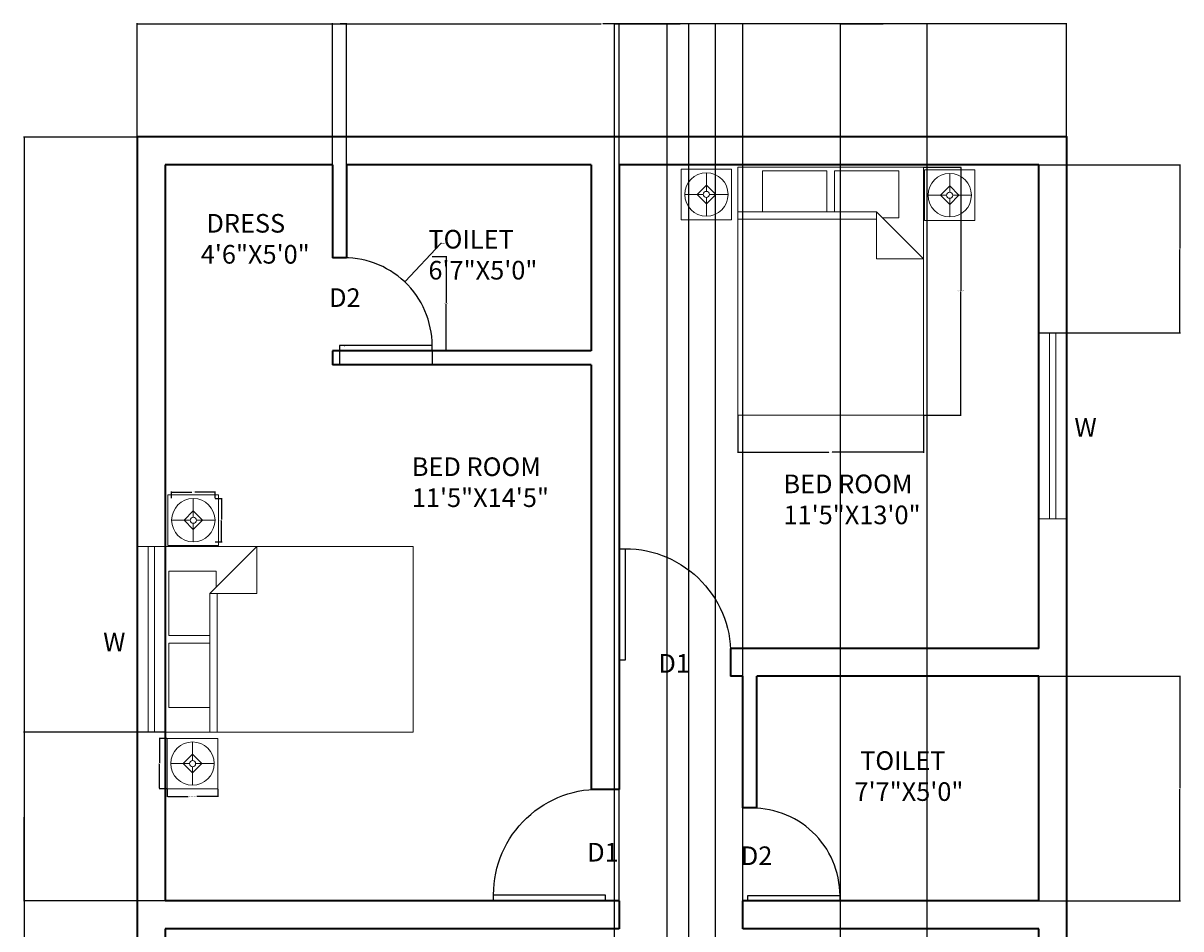
# Model space of a CAD drawing. Units: inches. Extents: x 2523 to 5630, y 2079 to 4208.
# Tile 3 of 3: x 2523 to 2897, y 2520 to 2812. Entities that reach past the tile are written whole.
import ezdxf

# ---------------------------------------------------------------- set-up
doc = ezdxf.new("R2010")
doc.units = ezdxf.units.IN
for name, color, linetype, lineweight in [('A-ANNO-DIMS', 2, 'Continuous', 18), ('A-ANNO-TEXT', 7, 'Continuous', 18), ('A-AREA-IDEN', 7, 'Continuous', 25), ('A-DOOR', 3, 'Continuous', 25), ('A-FURN', 8, 'Continuous', 18), ('A-GLAZ', 4, 'Continuous', 18), ('A-WALL', 7, 'Continuous', 35)]:
    doc.layers.add(name, color=color, linetype=linetype, lineweight=lineweight)
doc.styles.get("Standard").update_dxf_attribs({"font": 'arial.ttf'})
doc.dimstyles.get("Standard").update_dxf_attribs({"dimtxt": 0.18, "dimasz": 0.18, "dimexe": 0.18, "dimexo": 0.0625, "dimgap": 0.09, "dimtad": 0, "dimtih": 1, "dimtoh": 1, "dimdec": 4, "dimzin": 0, "dimdsep": 46, "dimtxsty": 'Standard', "dimcen": 0.09, "dimadec": 0, "dimazin": 0, "dimtfac": 1, "dimtdec": 4, "dimtofl": 0, "dimtmove": 0, "dimatfit": 3, "dimfxl": 1, "dimtolj": 1, "dimtzin": 0, "dimarcsym": 0})

# ---------------------------------------------------------------- blocks, each defined once
blk = doc.blocks.new('Bed - Queen')
for p, q in [((0, -80.00003), (0, 0)), ((0, 0), (59.99999, 0)), ((59.99999, 0), (59.99999, -80.00003)), ((7.99999, -1.2), (28.79998, -1.2)), ((7.99999, -14.4), (7.99999, -1.2)), ((28.79998, -1.2), (28.79998, -14.4)), ((31.19999, -1.2), (51.99999, -1.2)), ((31.19999, -14.4), (31.19999, -1.2)), ((51.99999, -1.2), (51.99999, -16.4)), ((0, -14.4), (44.8, -14.4)), ((59.99999, -29.6), (44.8, -14.4)), ((44.8, -14.4), (44.8, -29.6)), ((44.8, -16.8), (0, -16.8)), ((51.99999, -16.4), (46.79936, -16.4)), ((44.8, -29.6), (59.99999, -29.6)), ((59.99999, -80.00003), (0, -80.00003))]:
    blk.add_line(p, q)
blk = doc.blocks.new('Lamp - Table')
for p, q in [((0, 7), (0, 1)), ((-1, 0), (-7, 0)), ((0, 3), (-3, 0)), ((-3, 0), (0, -3)), ((3, 0), (0, 3)), ((0, -3), (3, 0)), ((1, 0), (7, 0)), ((0, -1), (0, -7))]:
    blk.add_line(p, q)
for radius in [7, 1]:
    blk.add_circle((0, 0), radius)
blk = doc.blocks.new('WIN-W-60IN')
for p, q in [((60, 5.5), (0, 5.5)), ((60, 3.5), (0, 3.5))]:
    blk.add_line(p, q)
blk.add_lwpolyline([(0, 0), (60, 0), (60, 9), (0, 9)], close=True)
blk = doc.blocks.new('DOOR-D1-36IN')
for p, q in [((2, 36), (0, 36)), ((2, 0), (2, 36)), ((0, 0), (2, 0))]:
    blk.add_line(p, q)
blk.add_arc((2, 34.06), 34.06, 270, 3.2732)
blk = doc.blocks.new('DOOR-D2-30IN')
for p, q in [((29.91, 1.66), (0, 1.66)), ((0, 1.66), (0, 0)), ((29.91, 0), (29.91, 1.66))]:
    blk.add_line(p, q)
blk.add_arc((1.62, 1.66), 28.29, 0, 93.2732)
blk = doc.blocks.new('TABLE-BEDSIDE')
blk.add_lwpolyline([(0, 0), (16.27, 0), (16.27, 16.36), (0, 16.36)], close=True)
blk = doc.blocks.new('*D16')
at = {"layer": 'A-ANNO-DIMS', "color": 0, "lineweight": -2, "transparency": 16777216}
for p, q in [((2813.56, 2765.62), (2825.68, 2765.62)), ((2825.5, 2765.44), (2825.5, 2725.81)), ((2825.5, 2685.8), (2825.5, 2725.43)), ((2813.56, 2685.62), (2825.68, 2685.62))]:
    blk.add_line(p, q, dxfattribs=at)
at = {"layer": 'A-ANNO-DIMS', "color": 0, "transparency": 16777216}
for points in [[(2825.47, 2765.44), (2825.53, 2765.44), (2825.5, 2765.62)], [(2825.47, 2685.8), (2825.53, 2685.8), (2825.5, 2685.62)]]:
    blk.add_solid(points, dxfattribs=at)
at = {"layer": 'Defpoints', "color": 0, "transparency": 16777216}
for p in [(2813.5, 2765.62), (2825.5, 2765.62), (2813.5, 2685.62)]:
    blk.add_point(p, dxfattribs=at)
at = {"layer": 'A-ANNO-DIMS', "color": 0, "transparency": 16777216, "insert": (2825.5, 2725.62), "char_height": 0.18, "attachment_point": 5}
blk.add_mtext('\\A1;QUEEN BED 80 TYP.', dxfattribs=at)
blk = doc.blocks.new('*D17')
at = {"layer": 'A-ANNO-DIMS', "color": 0, "lineweight": -2, "transparency": 16777216}
for p, q in [((2753.5, 2685.56), (2753.5, 2673.44)), ((2813.5, 2685.56), (2813.5, 2673.44)), ((2753.68, 2673.62), (2782.97, 2673.62)), ((2813.32, 2673.62), (2784.02, 2673.62))]:
    blk.add_line(p, q, dxfattribs=at)
at = {"layer": 'A-ANNO-DIMS', "color": 0, "transparency": 16777216}
for points in [[(2753.68, 2673.65), (2753.68, 2673.59), (2753.5, 2673.62)], [(2813.32, 2673.65), (2813.32, 2673.59), (2813.5, 2673.62)]]:
    blk.add_solid(points, dxfattribs=at)
at = {"layer": 'Defpoints', "color": 0, "transparency": 16777216}
for p in [(2753.5, 2685.62), (2813.5, 2685.62), (2813.5, 2673.62)]:
    blk.add_point(p, dxfattribs=at)
at = {"layer": 'A-ANNO-DIMS', "color": 0, "transparency": 16777216, "insert": (2783.5, 2673.62), "char_height": 0.18, "attachment_point": 5}
blk.add_mtext('\\A1;60 TYP.', dxfattribs=at)
blk = doc.blocks.new('*D18')
at = {"layer": 'A-ANNO-DIMS', "color": 0, "lineweight": -2, "transparency": 16777216}
for p, q in [((2569.34, 2564.95), (2569.34, 2562.38)), ((2585.7, 2564.95), (2585.7, 2562.38)), ((2569.52, 2562.56), (2576.13, 2562.56)), ((2585.52, 2562.56), (2578.9, 2562.56))]:
    blk.add_line(p, q, dxfattribs=at)
at = {"layer": 'A-ANNO-DIMS', "color": 0, "transparency": 16777216}
for points in [[(2569.52, 2562.59), (2569.52, 2562.53), (2569.34, 2562.56)], [(2585.52, 2562.59), (2585.52, 2562.53), (2585.7, 2562.56)]]:
    blk.add_solid(points, dxfattribs=at)
at = {"layer": 'Defpoints', "color": 0, "transparency": 16777216}
for p in [(2569.34, 2565.02), (2585.7, 2565.02), (2569.34, 2562.56)]:
    blk.add_point(p, dxfattribs=at)
at = {"layer": 'A-ANNO-DIMS', "color": 0, "transparency": 16777216, "insert": (2577.52, 2562.56), "char_height": 0.18, "attachment_point": 5}
blk.add_mtext('\\A1;NIGHT TABLE 16 TYP.', dxfattribs=at)
blk = doc.blocks.new('*D19')
at = {"layer": 'A-ANNO-DIMS', "color": 0, "lineweight": -2, "transparency": 16777216}
for p, q in [((2569.27, 2581.29), (2566.7, 2581.29)), ((2566.88, 2581.11), (2566.88, 2573.33)), ((2566.88, 2565.2), (2566.88, 2572.97)), ((2569.27, 2565.02), (2566.7, 2565.02))]:
    blk.add_line(p, q, dxfattribs=at)
at = {"layer": 'A-ANNO-DIMS', "color": 0, "transparency": 16777216}
for points in [[(2566.85, 2581.11), (2566.91, 2581.11), (2566.88, 2581.29)], [(2566.85, 2565.2), (2566.91, 2565.2), (2566.88, 2565.02)]]:
    blk.add_solid(points, dxfattribs=at)
at = {"layer": 'Defpoints', "color": 0, "transparency": 16777216}
for p in [(2566.88, 2581.29), (2569.34, 2581.29), (2569.34, 2565.02)]:
    blk.add_point(p, dxfattribs=at)
at = {"layer": 'A-ANNO-DIMS', "color": 0, "transparency": 16777216, "insert": (2566.88, 2573.15), "char_height": 0.18, "attachment_point": 5}
blk.add_mtext('\\A1;16 TYP.', dxfattribs=at)
blk = doc.blocks.new('*D20')
at = {"layer": 'A-ANNO-DIMS', "color": 0, "lineweight": -2, "transparency": 16777216}
for p, q in [((2584.83, 2658.68), (2587.05, 2658.68)), ((2586.87, 2658.5), (2586.87, 2651.86)), ((2586.87, 2644.86), (2586.87, 2651.5)), ((2584.83, 2644.68), (2587.05, 2644.68))]:
    blk.add_line(p, q, dxfattribs=at)
at = {"layer": 'A-ANNO-DIMS', "color": 0, "transparency": 16777216}
for points in [[(2586.84, 2658.5), (2586.9, 2658.5), (2586.87, 2658.68)], [(2586.84, 2644.86), (2586.9, 2644.86), (2586.87, 2644.68)]]:
    blk.add_solid(points, dxfattribs=at)
at = {"layer": 'Defpoints', "color": 0, "transparency": 16777216}
for p in [(2584.77, 2658.68), (2586.87, 2658.68), (2584.77, 2644.68)]:
    blk.add_point(p, dxfattribs=at)
at = {"layer": 'A-ANNO-DIMS', "color": 0, "transparency": 16777216, "insert": (2586.87, 2651.68), "char_height": 0.18, "attachment_point": 5}
blk.add_mtext('\\A1;LAMP 14 TYP.', dxfattribs=at)
blk = doc.blocks.new('*D21')
at = {"layer": 'A-ANNO-DIMS', "color": 0, "lineweight": -2, "transparency": 16777216}
for p, q in [((2570.77, 2658.75), (2570.77, 2660.96)), ((2584.77, 2658.75), (2584.77, 2660.96)), ((2570.95, 2660.78), (2577.25, 2660.78)), ((2584.59, 2660.78), (2578.29, 2660.78))]:
    blk.add_line(p, q, dxfattribs=at)
at = {"layer": 'A-ANNO-DIMS', "color": 0, "transparency": 16777216}
for points in [[(2570.95, 2660.81), (2570.95, 2660.75), (2570.77, 2660.78)], [(2584.59, 2660.81), (2584.59, 2660.75), (2584.77, 2660.78)]]:
    blk.add_solid(points, dxfattribs=at)
at = {"layer": 'Defpoints', "color": 0, "transparency": 16777216}
for p in [(2570.77, 2660.78), (2570.77, 2658.68), (2584.77, 2658.68)]:
    blk.add_point(p, dxfattribs=at)
at = {"layer": 'A-ANNO-DIMS', "color": 0, "transparency": 16777216, "insert": (2577.77, 2660.78), "char_height": 0.18, "attachment_point": 5}
blk.add_mtext('\\A1;14 TYP.', dxfattribs=at)
blk = doc.blocks.new('*D24')
at = {"layer": 'A-ANNO-DIMS', "color": 0, "lineweight": -2, "transparency": 16777216}
for p, q in [((2654.92, 2736.73), (2659.59, 2736.73)), ((2659.41, 2736.55), (2659.41, 2721.74)), ((2659.41, 2706.56), (2659.41, 2721.37)), ((2654.92, 2706.38), (2659.59, 2706.38))]:
    blk.add_line(p, q, dxfattribs=at)
at = {"layer": 'A-ANNO-DIMS', "color": 0, "transparency": 16777216}
for points in [[(2659.38, 2736.55), (2659.44, 2736.55), (2659.41, 2736.73)], [(2659.38, 2706.56), (2659.44, 2706.56), (2659.41, 2706.38)]]:
    blk.add_solid(points, dxfattribs=at)
at = {"layer": 'Defpoints', "color": 0, "transparency": 16777216}
for p in [(2654.86, 2736.73), (2659.41, 2736.73), (2654.86, 2706.38)]:
    blk.add_point(p, dxfattribs=at)
at = {"layer": 'A-ANNO-DIMS', "color": 0, "transparency": 16777216, "insert": (2659.41, 2721.56), "char_height": 0.18, "attachment_point": 5}
blk.add_mtext('\\A1;D2 30 TYP.', dxfattribs=at)
blk = doc.blocks.new('*D25')
at = {"layer": 'A-ANNO-DIMS', "color": 0, "lineweight": -2, "transparency": 16777216}
for p, q in [((2624.95, 2706.32), (2624.95, 2701.65)), ((2654.86, 2706.32), (2654.86, 2701.65)), ((2625.13, 2701.83), (2639.38, 2701.83)), ((2654.68, 2701.83), (2640.43, 2701.83))]:
    blk.add_line(p, q, dxfattribs=at)
at = {"layer": 'A-ANNO-DIMS', "color": 0, "transparency": 16777216}
for points in [[(2625.13, 2701.86), (2625.13, 2701.8), (2624.95, 2701.83)], [(2654.68, 2701.86), (2654.68, 2701.8), (2654.86, 2701.83)]]:
    blk.add_solid(points, dxfattribs=at)
at = {"layer": 'Defpoints', "color": 0, "transparency": 16777216}
for p in [(2624.95, 2706.38), (2654.86, 2706.38), (2654.86, 2701.83)]:
    blk.add_point(p, dxfattribs=at)
at = {"layer": 'A-ANNO-DIMS', "color": 0, "transparency": 16777216, "insert": (2639.9, 2701.83), "char_height": 0.18, "attachment_point": 5}
blk.add_mtext('\\A1;30 TYP.', dxfattribs=at)
blk = doc.blocks.new('*D32')
at = {"layer": 'A-ANNO-DIMS', "color": 0, "lineweight": -2, "transparency": 16777216}
for p, q in [((2559.69, 2775.4), (2559.69, 2812.06)), ((2559.87, 2811.88), (2709.4, 2811.88)), ((2859.51, 2811.88), (2709.98, 2811.88)), ((2859.69, 2775.4), (2859.69, 2812.06))]:
    blk.add_line(p, q, dxfattribs=at)
at = {"layer": 'A-ANNO-DIMS', "color": 0, "transparency": 16777216}
for points in [[(2559.87, 2811.91), (2559.87, 2811.85), (2559.69, 2811.88)], [(2859.51, 2811.91), (2859.51, 2811.85), (2859.69, 2811.88)]]:
    blk.add_solid(points, dxfattribs=at)
at = {"layer": 'Defpoints', "color": 0, "transparency": 16777216}
for p in [(2859.69, 2811.88), (2559.69, 2775.33), (2859.69, 2775.33)]:
    blk.add_point(p, dxfattribs=at)
at = {"layer": 'A-ANNO-DIMS', "color": 0, "transparency": 16777216, "insert": (2709.69, 2811.88), "char_height": 0.18, "attachment_point": 5}
blk.add_mtext('\\A1;300', dxfattribs=at)
blk = doc.blocks.new('*D33')
at = {"layer": 'A-ANNO-DIMS', "color": 0, "lineweight": -2, "transparency": 16777216}
for p, q in [((2559.63, 2775.33), (2522.96, 2775.33)), ((2523.14, 2775.15), (2523.14, 2445.52)), ((2523.14, 2115.51), (2523.14, 2445.15)), ((2559.63, 2115.33), (2522.96, 2115.33))]:
    blk.add_line(p, q, dxfattribs=at)
at = {"layer": 'A-ANNO-DIMS', "color": 0, "transparency": 16777216}
for points in [[(2523.11, 2775.15), (2523.17, 2775.15), (2523.14, 2775.33)], [(2523.11, 2115.51), (2523.17, 2115.51), (2523.14, 2115.33)]]:
    blk.add_solid(points, dxfattribs=at)
at = {"layer": 'Defpoints', "color": 0, "transparency": 16777216}
for p in [(2523.14, 2775.33), (2559.69, 2775.33), (2559.69, 2115.33)]:
    blk.add_point(p, dxfattribs=at)
at = {"layer": 'A-ANNO-DIMS', "color": 0, "transparency": 16777216, "insert": (2523.14, 2445.33), "char_height": 0.18, "attachment_point": 5}
blk.add_mtext('\\A1;660', dxfattribs=at)
blk = doc.blocks.new('*D40')
at = {"layer": 'A-ANNO-DIMS', "color": 0, "lineweight": -2, "transparency": 16777216}
for p, q in [((2786.69, 2195.9), (2786.69, 2812.06)), ((2786.87, 2811.88), (2800.47, 2811.88)), ((2814.51, 2811.88), (2800.91, 2811.88)), ((2814.69, 2195.9), (2814.69, 2812.06))]:
    blk.add_line(p, q, dxfattribs=at)
at = {"layer": 'A-ANNO-DIMS', "color": 0, "transparency": 16777216}
for points in [[(2786.87, 2811.91), (2786.87, 2811.85), (2786.69, 2811.88)], [(2814.51, 2811.91), (2814.51, 2811.85), (2814.69, 2811.88)]]:
    blk.add_solid(points, dxfattribs=at)
at = {"layer": 'Defpoints', "color": 0, "transparency": 16777216}
for p in [(2814.69, 2811.88), (2786.69, 2195.83), (2814.69, 2195.83)]:
    blk.add_point(p, dxfattribs=at)
at = {"layer": 'A-ANNO-DIMS', "color": 0, "transparency": 16777216, "insert": (2800.69, 2811.88), "char_height": 0.18, "attachment_point": 5}
blk.add_mtext('\\A1;28', dxfattribs=at)
blk = doc.blocks.new('*D41')
at = {"layer": 'A-ANNO-DIMS', "color": 0, "lineweight": -2, "transparency": 16777216}
for p, q in [((2730.69, 2160.15), (2730.69, 2812.06)), ((2730.87, 2811.88), (2734.04, 2811.88)), ((2737.51, 2811.88), (2734.34, 2811.88)), ((2737.69, 2160.15), (2737.69, 2812.06))]:
    blk.add_line(p, q, dxfattribs=at)
at = {"layer": 'A-ANNO-DIMS', "color": 0, "transparency": 16777216}
for points in [[(2730.87, 2811.91), (2730.87, 2811.85), (2730.69, 2811.88)], [(2737.51, 2811.91), (2737.51, 2811.85), (2737.69, 2811.88)]]:
    blk.add_solid(points, dxfattribs=at)
at = {"layer": 'Defpoints', "color": 0, "transparency": 16777216}
for p in [(2737.69, 2811.88), (2730.69, 2160.08), (2737.69, 2160.08)]:
    blk.add_point(p, dxfattribs=at)
at = {"layer": 'A-ANNO-DIMS', "color": 0, "transparency": 16777216, "insert": (2734.19, 2811.88), "char_height": 0.18, "attachment_point": 5}
blk.add_mtext('\\A1;7', dxfattribs=at)
blk = doc.blocks.new('*D42')
at = {"layer": 'A-ANNO-DIMS', "color": 0, "lineweight": -2, "transparency": 16777216}
for p, q in [((2850.76, 2766.33), (2896.42, 2766.33)), ((2896.24, 2766.15), (2896.24, 2739.4)), ((2896.24, 2712.28), (2896.24, 2739.03)), ((2850.76, 2712.1), (2896.42, 2712.1))]:
    blk.add_line(p, q, dxfattribs=at)
at = {"layer": 'A-ANNO-DIMS', "color": 0, "transparency": 16777216}
for points in [[(2896.21, 2766.15), (2896.27, 2766.15), (2896.24, 2766.33)], [(2896.21, 2712.28), (2896.27, 2712.28), (2896.24, 2712.1)]]:
    blk.add_solid(points, dxfattribs=at)
at = {"layer": 'Defpoints', "color": 0, "transparency": 16777216}
for p in [(2850.69, 2766.33), (2896.24, 2766.33), (2850.69, 2712.1)]:
    blk.add_point(p, dxfattribs=at)
at = {"layer": 'A-ANNO-DIMS', "color": 0, "transparency": 16777216, "insert": (2896.24, 2739.22), "char_height": 0.18, "attachment_point": 5}
blk.add_mtext('\\A1;54.24', dxfattribs=at)
blk = doc.blocks.new('*D45')
at = {"layer": 'A-ANNO-DIMS', "color": 0, "lineweight": -2, "transparency": 16777216}
for p, q in [((2568.63, 2583.25), (2522.96, 2583.25)), ((2523.14, 2583.07), (2523.14, 2556.22)), ((2523.14, 2529.01), (2523.14, 2555.86)), ((2568.63, 2528.83), (2522.96, 2528.83))]:
    blk.add_line(p, q, dxfattribs=at)
at = {"layer": 'A-ANNO-DIMS', "color": 0, "transparency": 16777216}
for points in [[(2523.11, 2583.07), (2523.17, 2583.07), (2523.14, 2583.25)], [(2523.11, 2529.01), (2523.17, 2529.01), (2523.14, 2528.83)]]:
    blk.add_solid(points, dxfattribs=at)
at = {"layer": 'Defpoints', "color": 0, "transparency": 16777216}
for p in [(2523.14, 2583.25), (2568.69, 2583.25), (2568.69, 2528.83)]:
    blk.add_point(p, dxfattribs=at)
at = {"layer": 'A-ANNO-DIMS', "color": 0, "transparency": 16777216, "insert": (2523.14, 2556.04), "char_height": 0.18, "attachment_point": 5}
blk.add_mtext('\\A1;54.41', dxfattribs=at)
blk = doc.blocks.new('*D49')
at = {"layer": 'A-ANNO-DIMS', "color": 0, "lineweight": -2, "transparency": 16777216}
for p, q in [((2713.69, 2204.9), (2713.69, 2812.06)), ((2713.87, 2811.88), (2729.54, 2811.88)), ((2746.14, 2811.88), (2730.47, 2811.88)), ((2746.32, 2204.9), (2746.32, 2812.06))]:
    blk.add_line(p, q, dxfattribs=at)
at = {"layer": 'A-ANNO-DIMS', "color": 0, "transparency": 16777216}
for points in [[(2713.87, 2811.91), (2713.87, 2811.85), (2713.69, 2811.88)], [(2746.14, 2811.91), (2746.14, 2811.85), (2746.32, 2811.88)]]:
    blk.add_solid(points, dxfattribs=at)
at = {"layer": 'Defpoints', "color": 0, "transparency": 16777216}
for p in [(2746.32, 2811.88), (2713.69, 2204.83), (2746.32, 2204.83)]:
    blk.add_point(p, dxfattribs=at)
at = {"layer": 'A-ANNO-DIMS', "color": 0, "transparency": 16777216, "insert": (2730.01, 2811.88), "char_height": 0.18, "attachment_point": 5}
blk.add_mtext('\\A1;32.625', dxfattribs=at)
blk = doc.blocks.new('*D50')
at = {"layer": 'A-ANNO-DIMS', "color": 0, "lineweight": -2, "transparency": 16777216}
for p, q in [((2850.76, 2601.33), (2896.42, 2601.33)), ((2896.24, 2601.15), (2896.24, 2565.27)), ((2896.24, 2529.01), (2896.24, 2564.9)), ((2850.76, 2528.83), (2896.42, 2528.83))]:
    blk.add_line(p, q, dxfattribs=at)
at = {"layer": 'A-ANNO-DIMS', "color": 0, "transparency": 16777216}
for points in [[(2896.21, 2601.15), (2896.27, 2601.15), (2896.24, 2601.33)], [(2896.21, 2529.01), (2896.27, 2529.01), (2896.24, 2528.83)]]:
    blk.add_solid(points, dxfattribs=at)
at = {"layer": 'Defpoints', "color": 0, "transparency": 16777216}
for p in [(2850.69, 2601.33), (2896.24, 2601.33), (2850.69, 2528.83)]:
    blk.add_point(p, dxfattribs=at)
at = {"layer": 'A-ANNO-DIMS', "color": 0, "transparency": 16777216, "insert": (2896.24, 2565.08), "char_height": 0.18, "attachment_point": 5}
blk.add_mtext('\\A1;72.5', dxfattribs=at)
blk = doc.blocks.new('*D51')
at = {"layer": 'A-ANNO-DIMS', "color": 0, "lineweight": -2, "transparency": 16777216}
for p, q in [((2715.19, 2519.9), (2715.19, 2812.06)), ((2715.37, 2811.88), (2734.97, 2811.88)), ((2755.01, 2811.88), (2735.42, 2811.88)), ((2755.19, 2519.9), (2755.19, 2812.06))]:
    blk.add_line(p, q, dxfattribs=at)
at = {"layer": 'A-ANNO-DIMS', "color": 0, "transparency": 16777216}
for points in [[(2715.37, 2811.91), (2715.37, 2811.85), (2715.19, 2811.88)], [(2755.01, 2811.91), (2755.01, 2811.85), (2755.19, 2811.88)]]:
    blk.add_solid(points, dxfattribs=at)
at = {"layer": 'Defpoints', "color": 0, "transparency": 16777216}
for p in [(2755.19, 2811.88), (2715.19, 2519.83), (2755.19, 2519.83)]:
    blk.add_point(p, dxfattribs=at)
at = {"layer": 'A-ANNO-DIMS', "color": 0, "transparency": 16777216, "insert": (2735.19, 2811.88), "char_height": 0.18, "attachment_point": 5}
blk.add_mtext('\\A1;40', dxfattribs=at)
blk = doc.blocks.new('*D52')
at = {"layer": 'A-ANNO-DIMS', "color": 0, "lineweight": -2, "transparency": 16777216}
for p, q in [((2622.69, 2766.4), (2622.69, 2812.06)), ((2622.87, 2811.88), (2624.68, 2811.88)), ((2627.01, 2811.88), (2625.2, 2811.88)), ((2627.19, 2766.4), (2627.19, 2812.06))]:
    blk.add_line(p, q, dxfattribs=at)
at = {"layer": 'A-ANNO-DIMS', "color": 0, "transparency": 16777216}
for points in [[(2622.87, 2811.91), (2622.87, 2811.85), (2622.69, 2811.88)], [(2627.01, 2811.91), (2627.01, 2811.85), (2627.19, 2811.88)]]:
    blk.add_solid(points, dxfattribs=at)
at = {"layer": 'Defpoints', "color": 0, "transparency": 16777216}
for p in [(2627.19, 2811.88), (2622.69, 2766.33), (2627.19, 2766.33)]:
    blk.add_point(p, dxfattribs=at)
at = {"layer": 'A-ANNO-DIMS', "color": 0, "transparency": 16777216, "insert": (2624.94, 2811.88), "char_height": 0.18, "attachment_point": 5}
blk.add_mtext('\\A1;4.5', dxfattribs=at)
blk = doc.blocks.new('*D55')
at = {"layer": 'A-ANNO-DIMS', "color": 0, "lineweight": -2, "transparency": 16777216}
for p, q in [((2657.65, 2740.95), (2646.12, 2728.74)), ((2657.83, 2740.95), (2657.65, 2740.95)), ((2626.47, 2708.04), (2626.65, 2708.04)), ((2626.56, 2707.95), (2626.56, 2708.13))]:
    blk.add_line(p, q, dxfattribs=at)
at = {"layer": 'A-ANNO-DIMS', "color": 0, "transparency": 16777216}
blk.add_solid([(2646.09, 2728.76), (2646.14, 2728.72), (2645.99, 2728.61)], dxfattribs=at)
at = {"layer": 'Defpoints', "color": 0, "transparency": 16777216}
for p in [(2645.99, 2728.61), (2626.56, 2708.04)]:
    blk.add_point(p, dxfattribs=at)
at = {"layer": 'A-ANNO-DIMS', "color": 0, "transparency": 16777216, "insert": (2658.57, 2740.95), "char_height": 0.18, "attachment_point": 5}
blk.add_mtext('\\A1;2X R28.294', dxfattribs=at)

msp = doc.modelspace()

# ---------------------------------------------------------------- linework, layer by layer
at = {"layer": 'A-DOOR'}
msp.add_line((2717.193, 2606.4881), (2715.193, 2606.4881), dxfattribs=at)
at = {"layer": 'A-WALL'}
for p, q in [((2568.693, 2766.334), (2568.693, 2528.834)), ((2622.693, 2766.334), (2568.693, 2766.334)), ((2622.693, 2766.334), (2622.693, 2736.3275)), ((2627.193, 2766.334), (2627.193, 2736.3275)), ((2706.193, 2766.334), (2627.193, 2766.334)), ((2706.193, 2766.334), (2706.193, 2706.334)), ((2850.693, 2766.334), (2715.193, 2766.334)), ((2715.193, 2766.334), (2715.193, 2564.834)), ((2850.693, 2610.334), (2850.693, 2766.334)), ((2627.193, 2736.3275), (2622.693, 2736.3275)), ((2627.193, 2706.334), (2622.693, 2706.334)), ((2622.693, 2706.334), (2622.693, 2701.834)), ((2706.193, 2706.334), (2627.193, 2706.334)), ((2706.193, 2701.834), (2622.693, 2701.834)), ((2706.193, 2701.834), (2706.193, 2564.834)), ((2850.693, 2610.334), (2751.193, 2610.334)), ((2751.193, 2610.334), (2751.193, 2601.334)), ((2755.193, 2601.334), (2751.193, 2601.334)), ((2755.193, 2558.834), (2755.193, 2601.334)), ((2850.693, 2601.334), (2759.693, 2601.334)), ((2759.693, 2558.834), (2759.693, 2601.334)), ((2850.693, 2528.834), (2850.693, 2601.334)), ((2715.193, 2564.834), (2706.193, 2564.834)), ((2759.693, 2558.834), (2755.193, 2558.834)), ((2715.193, 2528.834), (2568.693, 2528.834)), ((2715.193, 2528.834), (2715.193, 2519.834)), ((2850.693, 2528.834), (2755.193, 2528.834)), ((2755.193, 2519.834), (2755.193, 2528.834)), ((2715.193, 2519.834), (2568.693, 2519.834)), ((2568.693, 2519.834), (2568.693, 2357.834)), ((2850.693, 2519.834), (2755.193, 2519.834)), ((2850.693, 2357.834), (2850.693, 2519.834))]:
    msp.add_line(p, q, dxfattribs=at)
msp.add_lwpolyline([(2652.693, 2115.334), (2859.693, 2115.334), (2859.693, 2775.334), (2559.693, 2775.334), (2559.693, 2115.334), (2568.693, 2115.334)], dxfattribs=at)

# ---------------------------------------------------------------- block references
at = {"layer": 'A-DOOR'}
for p in [(2624.9494, 2706.3789), (2756.62, 2528.834)]:
    msp.add_blockref('DOOR-D2-30IN', p, dxfattribs=at)
at = {"layer": 'A-DOOR', "extrusion": (0, 0, -1), "zscale": -1}
for p, rotation in [((-2715.193, 2642.4881), 180), ((-2674.693, 2528.834), 90.00000000000138)]:
    msp.add_blockref('DOOR-D1-36IN', p, dxfattribs=dict(at, rotation=rotation))
at = {"layer": 'A-FURN'}
for name, p in [('Bed - Queen', (2753.4959, 2765.6208)), ('TABLE-BEDSIDE', (2735.2655, 2748.6181)), ('Lamp - Table', (2743.4003, 2756.7977)), ('TABLE-BEDSIDE', (2813.798, 2748.3658)), ('Lamp - Table', (2821.9327, 2756.5454))]:
    msp.add_blockref(name, p, dxfattribs=at)
for name, p, rotation in [('TABLE-BEDSIDE', (2585.9481, 2643.5487), 89.99999999999999), ('Lamp - Table', (2577.7685, 2651.6835), 90), ('Bed - Queen', (2568.693, 2583.2466), 90), ('TABLE-BEDSIDE', (2585.6958, 2565.0163), 90.00000000000266), ('Lamp - Table', (2577.5162, 2573.151), 90)]:
    msp.add_blockref(name, p, dxfattribs=dict(at, rotation=rotation))
at = {"layer": 'A-GLAZ'}
for p, rotation in [((2850.693, 2712.0974), 269.9999999999999), ((2559.693, 2643.2467), 269.9999999999993)]:
    msp.add_blockref('WIN-W-60IN', p, dxfattribs=dict(at, rotation=rotation))

# ---------------------------------------------------------------- texts
at = {"layer": 'A-ANNO-TEXT', "char_height": 6, "attachment_point": 1}
for s, insert in [('D2', (2621.5925, 2726.4969)), ('W', (2862.1969, 2684.6142)), ('W', (2548.6623, 2615.427)), ('D1', (2727.891, 2608.4772)), ('D1', (2704.9248, 2547.5574)), ('D2', (2754.5188, 2546.4143))]:
    msp.add_mtext_dynamic_manual_height_columns(s, width=48.58232, gutter_width=12.5, heights=[0], dxfattribs=dict(at, insert=insert))
at = {"layer": 'A-AREA-IDEN', "char_height": 6, "attachment_point": 1}
for s, insert in [(' DRESS\\P4\'6"X5\'0"', (2580.1662, 2750.4821)), ('TOILET\\P6\'7"X5\'0"', (2653.6576, 2745.3484)), ('BED ROOM\\P11\'5"X14\'5"', (2648.305, 2671.947)), ('BED ROOM\\P11\'5"X13\'0"', (2768.2696, 2666.3989)), (' TOILET\\P7\'7"X5\'0"', (2791.188, 2577.1194))]:
    msp.add_mtext_dynamic_manual_height_columns(s, width=48.58232, gutter_width=12.5, heights=[0], dxfattribs=dict(at, insert=insert))

# ---------------------------------------------------------------- dimensions: what is measured, and where the dimension line sits
at = {"layer": 'A-ANNO-DIMS'}
for base, p1, p2, override, picture, middle in [((2859.693, 2811.884), (2559.693, 2775.334), (2859.693, 2775.334), {"dimdec": 0, "dimlfac": 1, "dimrnd": 0, "dimzin": 0, "dimdsep": 46, "dimlunit": 2}, '*D32', (2709.693, 2811.884)), ((2627.193, 2811.884), (2622.693, 2766.334), (2627.193, 2766.334), {"dimdec": 1, "dimlfac": 1, "dimrnd": 0, "dimzin": 0, "dimdsep": 46, "dimlunit": 2}, '*D52', (2624.943, 2811.884)), ((2746.3179, 2811.884), (2713.693, 2204.834), (2746.3179, 2204.834), {"dimdec": 3, "dimlfac": 1, "dimrnd": 0, "dimzin": 0, "dimdsep": 46, "dimlunit": 2}, '*D49', (2730.0055, 2811.884)), ((2755.193, 2811.884), (2715.193, 2519.834), (2755.193, 2519.834), {"dimdec": 0, "dimlfac": 1, "dimrnd": 0, "dimzin": 0, "dimdsep": 46, "dimlunit": 2}, '*D51', (2735.193, 2811.884)), ((2737.693, 2811.884), (2730.693, 2160.084), (2737.693, 2160.084), {"dimdec": 0, "dimlfac": 1, "dimrnd": 0, "dimzin": 0, "dimdsep": 46, "dimlunit": 2}, '*D41', (2734.193, 2811.884)), ((2814.693, 2811.884), (2786.693, 2195.834), (2814.693, 2195.834), {"dimdec": 0, "dimlfac": 1, "dimrnd": 0, "dimzin": 0, "dimdsep": 46, "dimlunit": 2}, '*D40', (2800.693, 2811.884))]:
    dim = msp.add_linear_dim(base=base, p1=p1, p2=p2, dimstyle='Standard', override=override, dxfattribs=at)
    dim.commit()
    dim.dimension.update_dxf_attribs({"geometry": picture, "text_midpoint": middle})
for base, p1, p2, override, picture, middle in [((2523.143, 2775.334), (2559.693, 2115.334), (2559.693, 2775.334), {"dimdec": 0, "dimlfac": 1, "dimrnd": 0, "dimzin": 0, "dimdsep": 46, "dimlunit": 2}, '*D33', (2523.143, 2445.334)), ((2896.243, 2766.334), (2850.693, 2712.0973), (2850.693, 2766.334), {"dimdec": 2, "dimlfac": 1, "dimrnd": 0, "dimzin": 0, "dimdsep": 46, "dimlunit": 2}, '*D42', (2896.243, 2739.2157)), ((2896.243, 2601.334), (2850.693, 2528.834), (2850.693, 2601.334), {"dimdec": 1, "dimlfac": 1, "dimrnd": 0, "dimzin": 0, "dimdsep": 46, "dimlunit": 2}, '*D50', (2896.243, 2565.084)), ((2523.143, 2583.2466), (2568.693, 2528.834), (2568.693, 2583.2466), {"dimdec": 2, "dimlfac": 1, "dimrnd": 0, "dimzin": 0, "dimdsep": 46, "dimlunit": 2}, '*D45', (2523.143, 2556.0403))]:
    dim = msp.add_linear_dim(base=base, p1=p1, p2=p2, angle=90, dimstyle='Standard', override=override, dxfattribs=at)
    dim.commit()
    dim.dimension.update_dxf_attribs({"geometry": picture, "text_midpoint": middle})
for base, p1, p2, angle, text, picture, middle in [((2825.4959, 2765.6208), (2813.4959, 2685.6208), (2813.4959, 2765.6208), 90, 'QUEEN BED <> TYP.', '*D16', (2825.4959, 2725.6208)), ((2659.4114, 2736.7328), (2654.8583, 2706.379), (2654.8583, 2736.7328), 90, 'D2 <> TYP.', '*D24', (2659.4114, 2721.5559)), ((2570.7685, 2660.7835), (2584.7685, 2658.6835), (2570.7685, 2658.6835), 180, '<> TYP.', '*D21', (2577.7685, 2660.7835)), ((2586.8685, 2658.6835), (2584.7685, 2644.6835), (2584.7685, 2658.6835), 90, 'LAMP <> TYP.', '*D20', (2586.8685, 2651.6835)), ((2566.8825, 2581.2862), (2569.3364, 2565.0159), (2569.3364, 2581.2862), 90, '<> TYP.', '*D19', (2566.8825, 2573.151)), ((2569.3364, 2562.5619), (2585.6959, 2565.0159), (2569.3364, 2565.0159), 180, 'NIGHT TABLE <> TYP.', '*D18', (2577.5162, 2562.5619))]:
    dim = msp.add_linear_dim(base=base, p1=p1, p2=p2, angle=angle, text=text, dimstyle='Standard', override={"dimdec": 0, "dimlfac": 1, "dimrnd": 0, "dimzin": 0, "dimdsep": 46, "dimlunit": 2}, dxfattribs=at)
    dim.commit()
    dim.dimension.update_dxf_attribs({"geometry": picture, "text_midpoint": middle})
dim = msp.add_radius_dim(center=(2626.5645, 2708.0406), mpoint=(2645.9917, 2728.6106), text='2X <>', dimstyle='Standard', override={"dimdec": 3, "dimlfac": 1, "dimrnd": 0, "dimzin": 0, "dimdsep": 46, "dimlunit": 2}, dxfattribs=at)
dim.commit()
dim.dimension.update_dxf_attribs({"geometry": '*D55', "text_midpoint": (2658.5723, 2740.9527), "dimtype": 164})
for base, p1, p2, picture, middle in [((2654.8583, 2701.8259), (2624.949, 2706.379), (2654.8583, 2706.379), '*D25', (2639.9037, 2701.8259)), ((2813.4959, 2673.6208), (2753.4959, 2685.6208), (2813.4959, 2685.6208), '*D17', (2783.4959, 2673.6208))]:
    dim = msp.add_linear_dim(base=base, p1=p1, p2=p2, text='<> TYP.', dimstyle='Standard', override={"dimdec": 0, "dimlfac": 1, "dimrnd": 0, "dimzin": 0, "dimdsep": 46, "dimlunit": 2}, dxfattribs=at)
    dim.commit()
    dim.dimension.update_dxf_attribs({"geometry": picture, "text_midpoint": middle})

doc.saveas('drawing.dxf')
